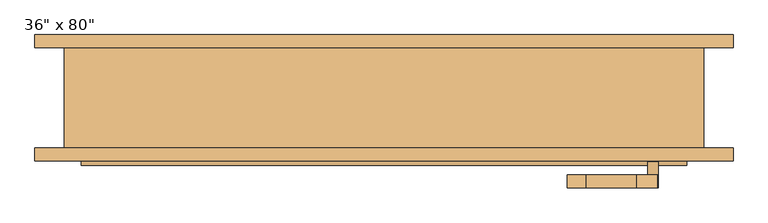
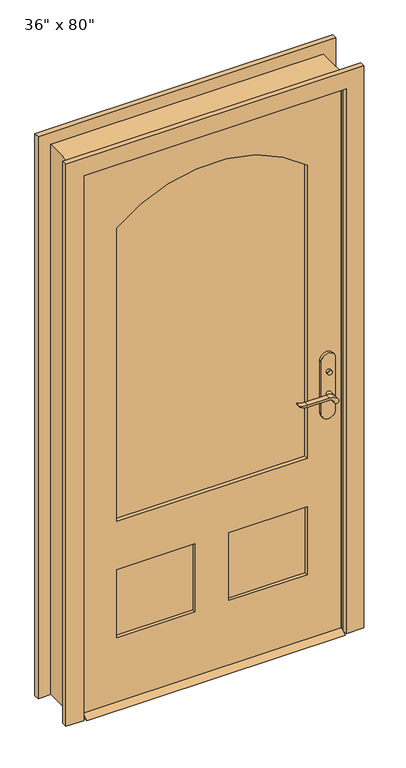
"""IFC4 building model written with IfcOpenShell, lengths in millimetres: door geometry."""

from ifc_helpers import new_model, si_unit, point, frame, frame_2d, origin, place, context, project, spatial, polyline, circle_curve, trimmed, segment, composite_curve, outline, extrude, faceted_brep, source, transform, mapped, element, save


def door_5d363d20(model_context):
    return source(origin(), model_context, "Body", "SolidModel", [
        extrude(outline(polyline([(-38.1, 12.7), (-12.7, 0.0), (-98.425, 0.0), (-73.025, 12.7), (-38.1, 12.7)])), frame((-457.2, 0.0, 0.0), z_axis=(1.0, 0.0, 0.0), x_axis=(0.0, 1.0, 0.0)), (0.0, 0.0, 1.0), 914.4),
        extrude(outline(polyline([(411.4, -18.1), (411.4, -28.1), (401.4, -28.1), (401.4, -18.1), (411.4, -18.1)])), frame((0.0, 0.0, 981.9), z_axis=(0.0, 0.0, 1.0), x_axis=(1.0, 0.0, 0.0)), (0.0, 0.0, 1.0), 30.0),
        extrude(outline(composite_curve([segment(trimmed(circle_curve(frame_2d((996.9, 406.4)), 8.0), [point((996.9, 398.4))], [point((996.9, 414.4))], False, "CARTESIAN"), True, "CONTINUOUS"), segment(trimmed(circle_curve(frame_2d((996.9, 406.4)), 8.0), [point((996.9, 414.4))], [point((996.9, 398.4))], False, "CARTESIAN"), True, "CONTINUOUS")], self_intersect=False)), frame((0.0, -93.025, 0.0), z_axis=(0.0, 1.0, 0.0), x_axis=(0.0, 0.0, 1.0)), (0.0, 0.0, 1.0), 10.0),
        extrude(outline(composite_curve([segment(trimmed(circle_curve(frame_2d((897.1555521, 382.7324871)), 37.2832219), [point((919.0523287, 412.9081363))], [point((934.4, 381.0325667))], False, "CARTESIAN"), True, "CONTINUOUS"), segment(polyline([(934.4, 381.0325667), (934.4, 304.7564091)]), True, "CONTINUOUS"), segment(trimmed(circle_curve(frame_2d((1017.6850638, 304.8227909)), 83.2850902), [point((934.4, 304.7564091))], [point((939.4, 276.4))], True, "CARTESIAN"), True, "CONTINUOUS"), segment(polyline([(939.4, 276.4), (936.6135558, 276.4)]), True, "CONTINUOUS"), segment(trimmed(circle_curve(frame_2d((986.6709207, 308.3396612)), 59.3791355), [point((936.6135558, 276.4))], [point((927.4, 304.7564091))], False, "CARTESIAN"), True, "CONTINUOUS"), segment(polyline([(927.4, 304.7564091), (927.4, 381.0138099)]), True, "CONTINUOUS"), segment(trimmed(circle_curve(frame_2d((909.2738613, 381.0138099)), 18.1261387), [point((927.4, 381.0138099))], [point((914.4, 398.4))], True, "CARTESIAN"), True, "CONTINUOUS"), segment(trimmed(circle_curve(frame_2d((914.4, 406.4)), 8.0), [point((914.4, 398.4))], [point((919.0523287, 412.9081363))], False, "CARTESIAN"), True, "CONTINUOUS")], self_intersect=False)), frame((0.0, 1.9, 0.0), z_axis=(0.0, 1.0, 0.0), x_axis=(0.0, 0.0, 1.0)), (0.0, 0.0, 1.0), 20.0),
        extrude(outline(composite_curve([segment(trimmed(circle_curve(frame_2d((914.4, 406.4)), 8.0), [point((914.3999903, 398.4))], [point((919.0523287, 412.9081363))], False, "CARTESIAN"), True, "CONTINUOUS"), segment(trimmed(circle_curve(frame_2d((897.1555521, 382.7324871)), 37.2832219), [point((919.0523287, 412.9081363))], [point((934.4, 381.0325667))], False, "CARTESIAN"), True, "CONTINUOUS"), segment(polyline([(934.4, 381.0325667), (934.4, 304.7564091)]), True, "CONTINUOUS"), segment(trimmed(circle_curve(frame_2d((1017.6850638, 304.8227909)), 83.2850902), [point((934.4, 304.7564091))], [point((939.4, 276.4))], True, "CARTESIAN"), True, "CONTINUOUS"), segment(polyline([(939.4, 276.4), (936.6135558, 276.4)]), True, "CONTINUOUS"), segment(trimmed(circle_curve(frame_2d((986.6709207, 308.3396612)), 59.3791355), [point((936.6135558, 276.4))], [point((927.4, 304.7564091))], False, "CARTESIAN"), True, "CONTINUOUS"), segment(polyline([(927.4, 304.7564091), (927.4, 381.0138122)]), True, "CONTINUOUS"), segment(trimmed(circle_curve(frame_2d((909.2738682, 381.0138122)), 18.1261318), [point((927.4, 381.0138122))], [point((914.3999903, 398.4))], True, "CARTESIAN"), True, "CONTINUOUS")], self_intersect=False)), frame((0.0, -133.025, 0.0), z_axis=(0.0, 1.0, 0.0), x_axis=(0.0, 0.0, 1.0)), (0.0, 0.0, 1.0), 20.0),
        extrude(outline(composite_curve([segment(trimmed(circle_curve(frame_2d((914.4, 406.4)), 8.0), [point((914.4, 398.4))], [point((914.4, 414.4))], False, "CARTESIAN"), True, "CONTINUOUS"), segment(trimmed(circle_curve(frame_2d((914.4, 406.4)), 8.0), [point((914.4, 414.4))], [point((914.4, 398.4))], False, "CARTESIAN"), True, "CONTINUOUS")], self_intersect=False)), frame((0.0, -28.1, 0.0), z_axis=(0.0, 1.0, 0.0), x_axis=(0.0, 0.0, 1.0)), (0.0, 0.0, 1.0), 30.0),
        extrude(outline(composite_curve([segment(trimmed(circle_curve(frame_2d((914.4, 406.4)), 8.0), [point((914.4, 398.4))], [point((914.4, 414.4))], False, "CARTESIAN"), True, "CONTINUOUS"), segment(trimmed(circle_curve(frame_2d((914.4, 406.4)), 8.0), [point((914.4, 414.4))], [point((914.4, 398.4))], False, "CARTESIAN"), True, "CONTINUOUS")], self_intersect=False)), frame((0.0, -113.025, 0.0), z_axis=(0.0, 1.0, 0.0), x_axis=(0.0, 0.0, 1.0)), (0.0, 0.0, 1.0), 30.0),
        extrude(outline(composite_curve([segment(polyline([(844.4, 431.4), (1039.4, 431.4)]), True, "CONTINUOUS"), segment(trimmed(circle_curve(frame_2d((1039.4, 406.4)), 25.0), [point((1039.4, 431.4))], [point((1039.4, 381.4))], False, "CARTESIAN"), True, "CONTINUOUS"), segment(polyline([(1039.4, 381.4), (844.4, 381.4)]), True, "CONTINUOUS"), segment(trimmed(circle_curve(frame_2d((844.4, 406.4)), 25.0), [point((844.4, 381.4))], [point((844.4, 431.4))], False, "CARTESIAN"), True, "CONTINUOUS")], self_intersect=False)), frame((0.0, -38.1, 0.0), z_axis=(0.0, 1.0, 0.0), x_axis=(0.0, 0.0, 1.0)), (0.0, 0.0, 1.0), 10.0),
        extrude(outline(composite_curve([segment(polyline([(844.4, 431.4), (1039.4, 431.4)]), True, "CONTINUOUS"), segment(trimmed(circle_curve(frame_2d((1039.4, 406.4)), 25.0), [point((1039.4, 431.4))], [point((1039.4, 381.4))], False, "CARTESIAN"), True, "CONTINUOUS"), segment(polyline([(1039.4, 381.4), (844.4, 381.4)]), True, "CONTINUOUS"), segment(trimmed(circle_curve(frame_2d((844.4, 406.4)), 25.0), [point((844.4, 381.4))], [point((844.4, 431.4))], False, "CARTESIAN"), True, "CONTINUOUS")], self_intersect=False)), frame((0.0, -83.025, 0.0), z_axis=(0.0, 1.0, 0.0), x_axis=(0.0, 0.0, 1.0)), (0.0, 0.0, 1.0), 10.0),
        extrude(outline(polyline([(2032.0, -457.2), (12.7, -457.2), (12.7, 457.2), (2032.0, 457.2), (2032.0, -457.2)]), holes=[composite_curve([segment(polyline([(688.975, -336.55), (1784.35, -336.55)]), True, "CONTINUOUS"), segment(trimmed(circle_curve(frame_2d((1401.92125, 0.0)), 509.42875), [point((1784.35, -336.55))], [point((1784.35, 336.55))], True, "CARTESIAN"), True, "CONTINUOUS"), segment(polyline([(1784.35, 336.55), (688.975, 336.55), (688.975, -336.55)]), True, "CONTINUOUS")], self_intersect=False), polyline([(508.0, -60.325), (254.0, -60.325), (254.0, -336.55), (508.0, -336.55), (508.0, -60.325)]), polyline([(508.0, 336.55), (254.0, 336.55), (254.0, 60.325), (508.0, 60.325), (508.0, 336.55)])]), frame((0.0, -73.025, 0.0), z_axis=(0.0, 1.0, 0.0), x_axis=(0.0, 0.0, 1.0)), (0.0, 0.0, 1.0), 34.925),
        faceted_brep([(482.6, -73.025, 0.0), (457.2, -73.025, 0.0), (457.2, -38.1, 0.0), (444.5, -38.1, 0.0), (444.5, -3.175, 0.0), (457.2, -3.175, 0.0), (457.2, 79.375, 0.0), (482.6, 79.375, 0.0), (482.6, 79.375, 2057.4), (482.6, -73.025, 2057.4), (457.2, 79.375, 2032.0), (-457.2, 79.375, 2032.0), (-457.2, 79.375, 0.0), (-482.6, 79.375, 0.0), (-482.6, 79.375, 2057.4), (457.2, -3.175, 2032.0), (444.5, -3.175, 2019.3), (-444.5, -3.175, 2019.3), (-444.5, -3.175, 0.0), (-457.2, -3.175, 0.0), (-457.2, -3.175, 2032.0), (444.5, -38.1, 2019.3), (457.2, -38.1, 2032.0), (-457.2, -38.1, 2032.0), (-457.2, -38.1, 0.0), (-444.5, -38.1, 0.0), (-444.5, -38.1, 2019.3), (457.2, -73.025, 2032.0), (-482.6, -73.025, 2057.4), (-482.6, -73.025, 0.0), (-457.2, -73.025, 0.0), (-457.2, -73.025, 2032.0)], [[[0, 1, 2, 3, 4, 5, 6, 7]], [[7, 8, 9, 0]], [[6, 10, 11, 12, 13, 14, 8, 7]], [[5, 15, 10, 6]], [[4, 16, 17, 18, 19, 20, 15, 5]], [[3, 21, 16, 4]], [[2, 22, 23, 24, 25, 26, 21, 3]], [[1, 27, 22, 2]], [[0, 9, 28, 29, 30, 31, 27, 1]], [[8, 14, 28, 9]], [[15, 20, 11, 10]], [[21, 26, 17, 16]], [[27, 31, 23, 22]], [[29, 13, 12, 19, 18, 25, 24, 30]], [[14, 13, 29, 28]], [[20, 19, 12, 11]], [[26, 25, 18, 17]], [[31, 30, 24, 23]]]),
        extrude(outline(polyline([(-60.325, -49.7416667), (-60.325, -61.3833333), (-336.55, -61.3833333), (-336.55, -49.7416667), (-60.325, -49.7416667)])), frame((0.0, 0.0, 254.0), z_axis=(0.0, 0.0, 1.0), x_axis=(1.0, 0.0, 0.0)), (0.0, 0.0, 1.0), 254.0),
        extrude(outline(polyline([(336.55, -49.7416667), (336.55, -61.3833333), (60.325, -61.3833333), (60.325, -49.7416667), (336.55, -49.7416667)])), frame((0.0, 0.0, 254.0), z_axis=(0.0, 0.0, 1.0), x_axis=(1.0, 0.0, 0.0)), (0.0, 0.0, 1.0), 254.0),
        extrude(outline(composite_curve([segment(polyline([(688.975, -336.55), (688.975, 336.55), (1784.35, 336.55)]), True, "CONTINUOUS"), segment(trimmed(circle_curve(frame_2d((1401.92125, 0.0)), 509.42875), [point((1784.35, 336.55))], [point((1784.35, -336.55))], False, "CARTESIAN"), True, "CONTINUOUS"), segment(polyline([(1784.35, -336.55), (688.975, -336.55)]), True, "CONTINUOUS")], self_intersect=False)), frame((0.0, -59.055, 0.0), z_axis=(0.0, 1.0, 0.0), x_axis=(0.0, 0.0, 1.0)), (0.0, 0.0, 1.0), 6.985),
        extrude(outline(polyline([(0.0, -463.55), (2038.35, -463.55), (2038.35, 463.55), (0.0, 463.55), (0.0, 527.05), (2101.85, 527.05), (2101.85, -527.05), (0.0, -527.05), (0.0, -463.55)])), frame((0.0, 79.375, 0.0), z_axis=(0.0, 1.0, 0.0), x_axis=(0.0, 0.0, 1.0)), (0.0, 0.0, 1.0), 19.05),
        extrude(outline(polyline([(0.0, -463.55), (2038.35, -463.55), (2038.35, 463.55), (0.0, 463.55), (0.0, 527.05), (2101.85, 527.05), (2101.85, -527.05), (0.0, -527.05), (0.0, -463.55)])), frame((0.0, -92.075, 0.0), z_axis=(0.0, 1.0, 0.0), x_axis=(0.0, 0.0, 1.0)), (0.0, 0.0, 1.0), 19.05),
    ])


if __name__ == "__main__":
    model = new_model("IFC4")
    model_context = context("Model", 3, world=origin())
    ifc_project = project(units=[si_unit("LENGTHUNIT", "METRE", prefix="MILLI")], contexts=[model_context])
    site = spatial("IfcSite", under=ifc_project)
    building = spatial("IfcBuilding", under=site)
    placement = place(None, origin())
    door_shape = door_5d363d20(model_context)
    element("IfcDoor", 1, ObjectType="36\" x 80\"", at=placement, inside=building, context=model_context, shape_type="MappedRepresentation", body=[
        mapped(door_shape, transform((0.0, 0.0, 0.0), x_axis=(1.0, 0.0, 0.0), y_axis=(0.0, 1.0, 0.0), z_axis=(0.0, 0.0, 1.0))),
    ])
    save(model, "model.ifc")

# Revit data of these elements
# Type "36\" x 80\""
#   Type Mark = "8"
#   Assembly Code = "B2030100"
#   Analytic Construction = "French door, wood frame with single glass"
#   Threshold Offset [instance default] = 0' - 0 1/2"
#   Thickness = 0' - 1 3/8"
#   Thermal Resistance (R) = 1.0696 (h·ft²·°F)/BTU
#   Swing Angle [instance default] = 90.00°
#   Stiles = 0' - 4 3/4"
#   Rough Width = 3' - 2"
#   Rough Height = 6' - 9"
#   Radius = 1' - 8.05625"
#   Lock Rail = 0' - 7 1/8"
#   Height = 6' - 8"
#   Width = 3' - 0"
#   Heat Transfer Coefficient (U) = 0.9350 BTU/(h·ft²·°F)
#   Door Offset [instance default] = 0' - 0"
#   Bottom Rail = 0' - 9 1/2"
#   Threshold [instance default] = yes
#   Function = 1
#   Exterior Trim [instance default] = yes
#   Trim Material = Cherry
#   Threshold Material = Cherry
#   Panel Material = Cherry
#   Glazing = Glass
#   Frame Material = Cherry
#   Door Handle Material = Aluminum
#   Visual Light Transmittance = 0
#   Solar Heat Gain Coefficient = 0
#   Wall Closure = (empty or 0)
#   Construction Type = (empty or 0)
# Element 1 (IfcDoor, "36\" x 80\"")
#   Materials on its faces: "Cherry", "Aluminum", "Glass"
# Materials
#   "Cherry": class "Wood", colour RGB 226 177 128, transparency 0, Description = "Prunus Serotina", Cost = 0
#   "Glass": class "Glass", colour RGB 0 128 192, transparency 0.75, Description = "Soda Lime Glass", Cost = 0
#   "Aluminum": class "Metal", colour RGB 247 247 247, transparency 0, Description = "Aluminum 6061", Cost = 0
